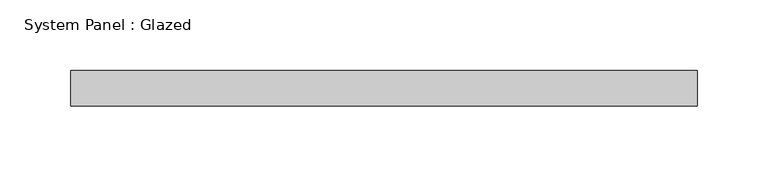
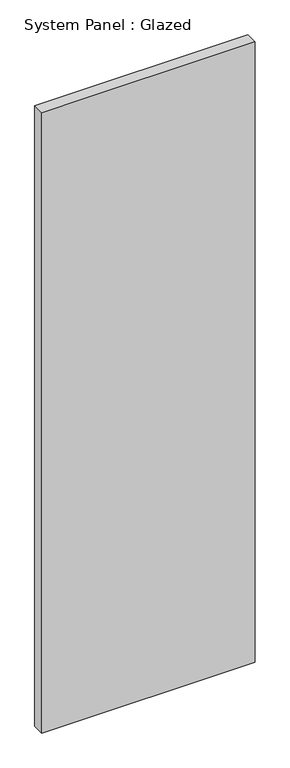
"""IFC4 building model written with IfcOpenShell, lengths in millimetres: plate geometry, System Panel : Glazed."""

from ifc_helpers import new_model, si_unit, origin, origin_with_axes, place, context, project, spatial, polyline, outline, extrude, source, transform, mapped, element, save


def system_panel_glazed_d4ab74e0(model_context):
    return source(origin(), model_context, "Body", "SweptSolid", [
        extrude(outline(polyline([(222.25, 19.05), (-222.25, 19.05), (-222.25, 44.45), (222.25, 44.45), (222.25, 19.05)])), origin_with_axes(), (0.0, 0.0, 1.0), 1367.7499719),
    ])


if __name__ == "__main__":
    model = new_model("IFC4")
    model_context = context("Model", 3, world=origin())
    ifc_project = project(units=[si_unit("LENGTHUNIT", "METRE", prefix="MILLI")], contexts=[model_context])
    site = spatial("IfcSite", under=ifc_project)
    building = spatial("IfcBuilding", under=site)
    placement = place(None, origin())
    system_panel_glazed_shape = system_panel_glazed_d4ab74e0(model_context)
    element("IfcPlate", 1, ObjectType="System Panel : Glazed", at=placement, inside=building, context=model_context, shape_type="MappedRepresentation", body=[
        mapped(system_panel_glazed_shape, transform((0.0, 0.0, 0.0), x_axis=(1.0, 0.0, 0.0), y_axis=(0.0, 1.0, 0.0), z_axis=(0.0, 0.0, 1.0))),
    ])
    save(model, "model.ifc")

# Revit data of these elements
# Type "System Panel : Glazed"
#   Construction Type Id = "GSP4R"
#   Analytic Construction = "1/8 in Pilkington single glazing"
#   Visual Light Transmittance = 0.9
#   Solar Heat Gain Coefficient = 0.86
#   Heat Transfer Coefficient (U) = 1.18115 BTU/(h·ft²·°F)
#   Define Thermal Properties by = 1
# Element 1 (IfcPlate, "System Panel : Glazed")
#   Materials on its faces: "Glass"
# Materials
#   "Glass": class "Glass", colour RGB 0 128 192, transparency 0.75, Description = "Soda Lime Glass", Cost = 0
